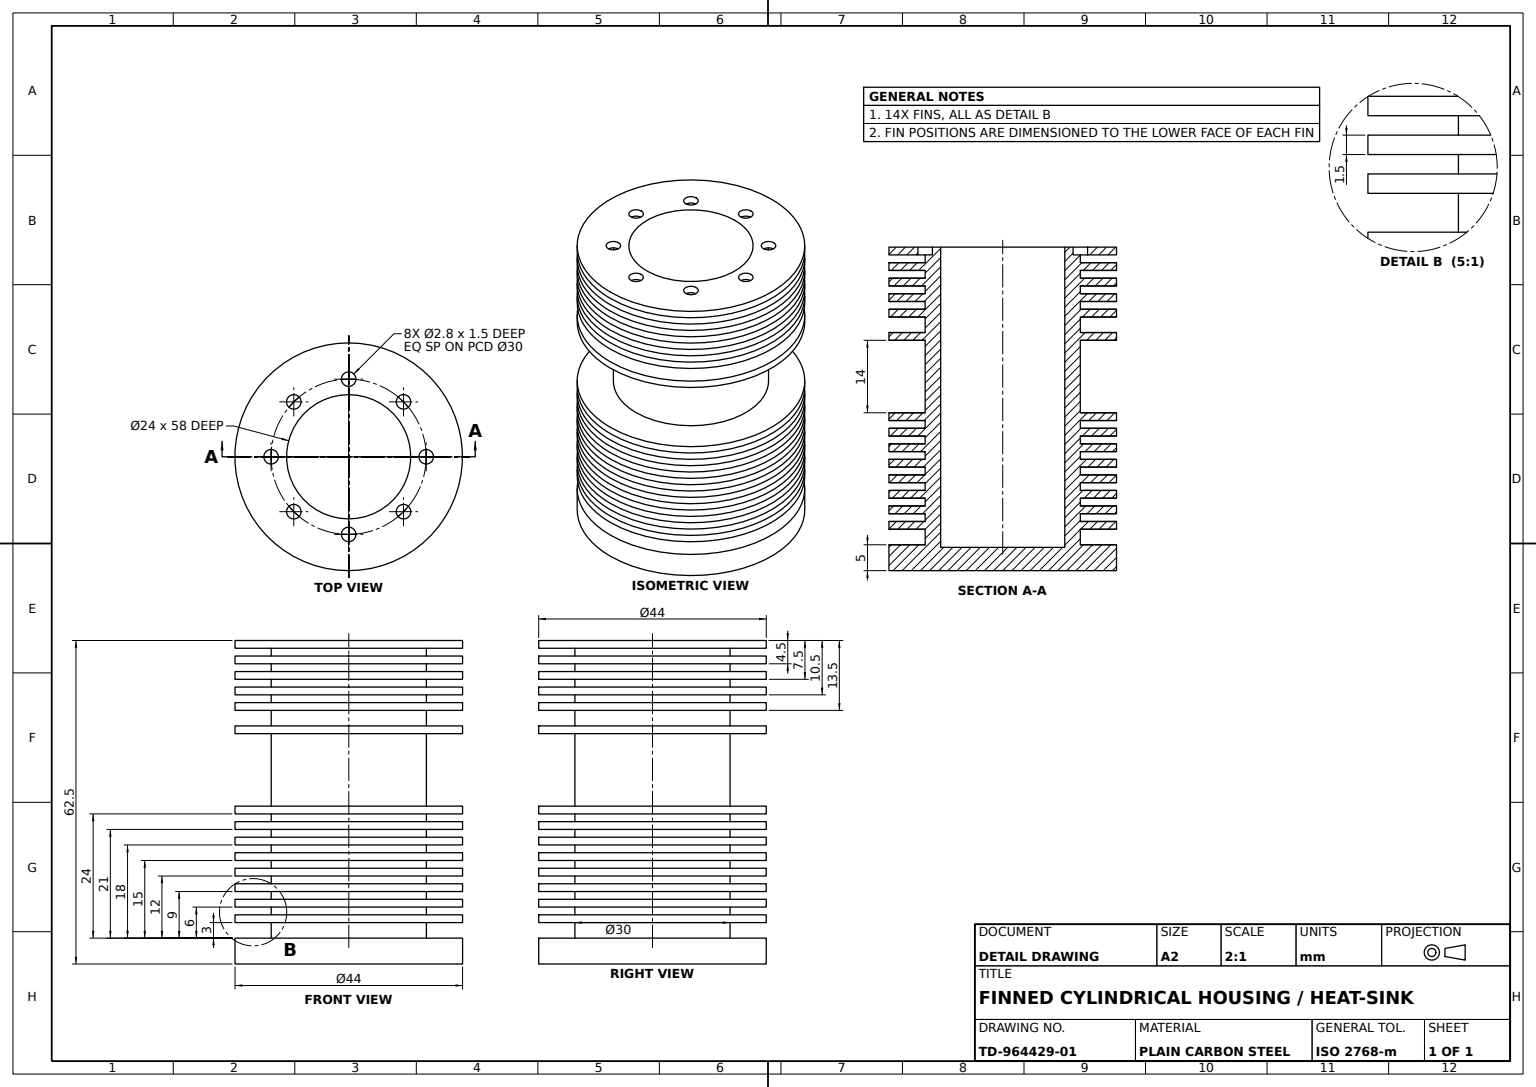
SolidWorks part; units mm, degrees
material "Plain Carbon Steel"
ref_plane "Front Plane" through (0, 0, 0) normal (0, 0, 1) x (1, 0, 0)
ref_plane "Top Plane" through (0, 0, 0) normal (0, 1, 0) x (1, 0, 0)
ref_plane "Right Plane" through (0, 0, 0) normal (1, 0, 0) x (0, 0, -1)
sketch "Base Disc Sketch" plane through (0, 0, 0) normal (0, 1, 0) x (1, 0, 0)
  circle A0 centre (0, 0) radius 22
  dimension "D1" = 44
extrude "Base Disc" add sketch "Base Disc Sketch" along normal blind 5
ref_plane "Lower Fin 1 Plane" through (0, 8, 0) normal (0, 1, 0) x (1, 0, 0)
ref_plane "Lower Fin 2 Plane" through (0, 11, 0) normal (0, 1, 0) x (1, 0, 0)
ref_plane "Lower Fin 3 Plane" through (0, 14, 0) normal (0, 1, 0) x (1, 0, 0)
ref_plane "Lower Fin 4 Plane" through (0, 17, 0) normal (0, 1, 0) x (1, 0, 0)
ref_plane "Lower Fin 5 Plane" through (0, 20, 0) normal (0, 1, 0) x (1, 0, 0)
ref_plane "Lower Fin 6 Plane" through (0, 23, 0) normal (0, 1, 0) x (1, 0, 0)
ref_plane "Lower Fin 7 Plane" through (0, 26, 0) normal (0, 1, 0) x (1, 0, 0)
ref_plane "Lower Fin 8 Plane" through (0, 29, 0) normal (0, 1, 0) x (1, 0, 0)
sketch "Lower Fin 1 Sketch" plane through (0, 8, 0) normal (0, 1, 0) x (1, 0, 0)
  circle A0 centre (0, 0) radius 22 construction
  circle A1 centre (0, 0) radius 22
sketch "Lower Fin 2 Sketch" plane through (0, 11, 0) normal (0, 1, 0) x (1, 0, 0)
  circle A0 centre (0, 0) radius 22 construction
  circle A1 centre (0, 0) radius 22
sketch "Lower Fin 3 Sketch" plane through (0, 14, 0) normal (0, 1, 0) x (1, 0, 0)
  circle A1 centre (0, 0) radius 22
  circle A2 centre (0, 0) radius 22
  dimension "D1" = 0
sketch "Lower Fin 4 Sketch" plane through (0, 17, 0) normal (0, 1, 0) x (1, 0, 0)
  circle A0 centre (0, 0) radius 22 construction
  circle A1 centre (0, 0) radius 22
sketch "Lower Fin 5 Sketch" plane through (0, 20, 0) normal (0, 1, 0) x (1, 0, 0)
  circle A0 centre (0, 0) radius 22 construction
  circle A1 centre (0, 0) radius 22
sketch "Lower Fin 6 Sketch" plane through (0, 23, 0) normal (0, 1, 0) x (1, 0, 0)
  circle A0 centre (0, 0) radius 22 construction
  circle A1 centre (0, 0) radius 22
sketch "Lower Fin 7 Sketch" plane through (0, 26, 0) normal (0, 1, 0) x (1, 0, 0)
  circle A1 centre (0, 0) radius 22
  circle A2 centre (0, 0) radius 22
  dimension "D1" = 0
sketch "Lower Fin 8 Sketch" plane through (0, 29, 0) normal (0, 1, 0) x (1, 0, 0)
  circle A0 centre (0, 0) radius 22 construction
  circle A1 centre (0, 0) radius 22
extrude "Lower Fin 1" add sketch "Lower Fin 1 Sketch" along normal blind 1.5 separate body contours A1
extrude "Lower Fin 2" add sketch "Lower Fin 2 Sketch" along normal blind 1.5 separate body contours A1
extrude "Lower Fin 3" add sketch "Lower Fin 3 Sketch" along normal blind 1.5 separate body contours A2
extrude "Lower Fin 4" add sketch "Lower Fin 4 Sketch" along normal blind 1.5 separate body contours A1
extrude "Lower Fin 5" add sketch "Lower Fin 5 Sketch" along normal blind 1.5 separate body contours A1
extrude "Lower Fin 6" add sketch "Lower Fin 6 Sketch" along normal blind 1.5 separate body contours A1
extrude "Lower Fin 7" add sketch "Lower Fin 7 Sketch" along normal blind 1.5 separate body contours A2
extrude "Lower Fin 8" add sketch "Lower Fin 8 Sketch" along normal blind 1.5 separate body contours A1
ref_plane "Upper Fin 1 Plane" through (0, 44.5, 0) normal (0, 1, 0) x (1, 0, 0)
sketch "Upper Fin 1 Sketch" plane through (0, 44.5, 0) normal (0, 1, 0) x (1, 0, 0)
  circle A0 centre (0, 0) radius 22 construction
  circle A1 centre (0, 0) radius 22
extrude "Upper Fin 1" add sketch "Upper Fin 1 Sketch" along normal blind 1.5 separate body
ref_plane "Upper Fin 2 Plane" through (0, 49, 0) normal (0, 1, 0) x (1, 0, 0)
ref_plane "Upper Fin 3 Plane" through (0, 52, 0) normal (0, 1, 0) x (1, 0, 0)
ref_plane "Upper Fin 4 Plane" through (0, 55, 0) normal (0, 1, 0) x (1, 0, 0)
ref_plane "Upper Fin 5 Plane" through (0, 58, 0) normal (0, 1, 0) x (1, 0, 0)
ref_plane "Upper Fin 6 Plane" through (0, 61, 0) normal (0, 1, 0) x (1, 0, 0)
sketch "Upper Fin 2 Sketch" plane through (0, 49, 0) normal (0, 1, 0) x (1, 0, 0)
  circle A0 centre (0, 0) radius 22 construction
  circle A1 centre (0, 0) radius 22
extrude "Upper Fin 2" add sketch "Upper Fin 2 Sketch" along normal blind 1.5 separate body
sketch "Upper Fin 3 Sketch" plane through (0, 52, 0) normal (0, 1, 0) x (1, 0, 0)
  circle A0 centre (0, 0) radius 22 construction
  circle A1 centre (0, 0) radius 22
extrude "Upper Fin 3" add sketch "Upper Fin 3 Sketch" along normal blind 1.5 separate body
sketch "Upper Fin 4 Sketch" plane through (0, 55, 0) normal (0, 1, 0) x (1, 0, 0)
  circle A0 centre (0, 0) radius 22 construction
  circle A1 centre (0, 0) radius 22
extrude "Upper Fin 4" add sketch "Upper Fin 4 Sketch" along normal blind 1.5 separate body
sketch "Upper Fin 5 Sketch" plane through (0, 58, 0) normal (0, 1, 0) x (1, 0, 0)
  circle A0 centre (0, 0) radius 22 construction
  circle A1 centre (0, 0) radius 22
extrude "Upper Fin 5" add sketch "Upper Fin 5 Sketch" along normal blind 1.5 separate body
sketch "Upper Fin 6 Sketch" plane through (0, 61, 0) normal (0, 1, 0) x (1, 0, 0)
  circle A1 centre (0, 0) radius 22
  circle A2 centre (0, 0) radius 22
  dimension "D1" = 0
extrude "Upper Fin 6" add sketch "Upper Fin 6 Sketch" along normal blind 1.5 separate body
sketch "Core Boss Sketch" plane through (0, 62.5, 0) normal (0, 1, 0) x (1, 0, 0)
  circle A0 centre (0, 0) radius 12
  dimension "D1" = 24
extrude "Core Boss 58mm" add sketch "Core Boss Sketch" against normal blind 58
sketch "Hub Boss Sketch" plane through (0, 62.5, 0) normal (0, 1, 0) x (1, 0, 0)
  circle A0 centre (0, 0) radius 15
  dimension "D1" = 30
extrude "Hub Boss 58mm" add sketch "Hub Boss Sketch" against normal blind 58
sketch "Central Bore Sketch" plane through (0, 62.5, 0) normal (0, 1, 0) x (1, 0, 0)
  circle A0 centre (0, 0) radius 12
  dimension "D1" = 24
extrude "Central Bore" cut sketch "Central Bore Sketch" against normal blind 58
sketch "Bolt Holes 8x Sketch" plane through (0, 62.5, 0) normal (0, 1, 0) x (1, 0, 0)
  circle A1 centre (0, 15) radius 1.4
  circle A2 centre (10.6066, 10.6066) radius 1.4
  circle A3 centre (15, 0) radius 1.4
  circle A4 centre (10.6066, -10.6066) radius 1.4
  circle A5 centre (0, -15) radius 1.4
  circle A6 centre (-10.6066, -10.6066) radius 1.4
  circle A7 centre (-15, 0) radius 1.4
  circle A8 centre (-10.6066, 10.6066) radius 1.4
  circle A9 centre (0, 0) radius 12 construction
  dimension "D1" = 8
  dimension "D2" = 2.8
  dimension "D3" = 10.6066
  dimension "D4" = 15
  dimension "D5" = 10.6066
extrude "Bolt Holes 8x" cut sketch "Bolt Holes 8x Sketch" against normal blind 1.5
ref_plane "Plane15" through (15, 0, 0) normal (1, 0, 0) x (0, 0, -1)
